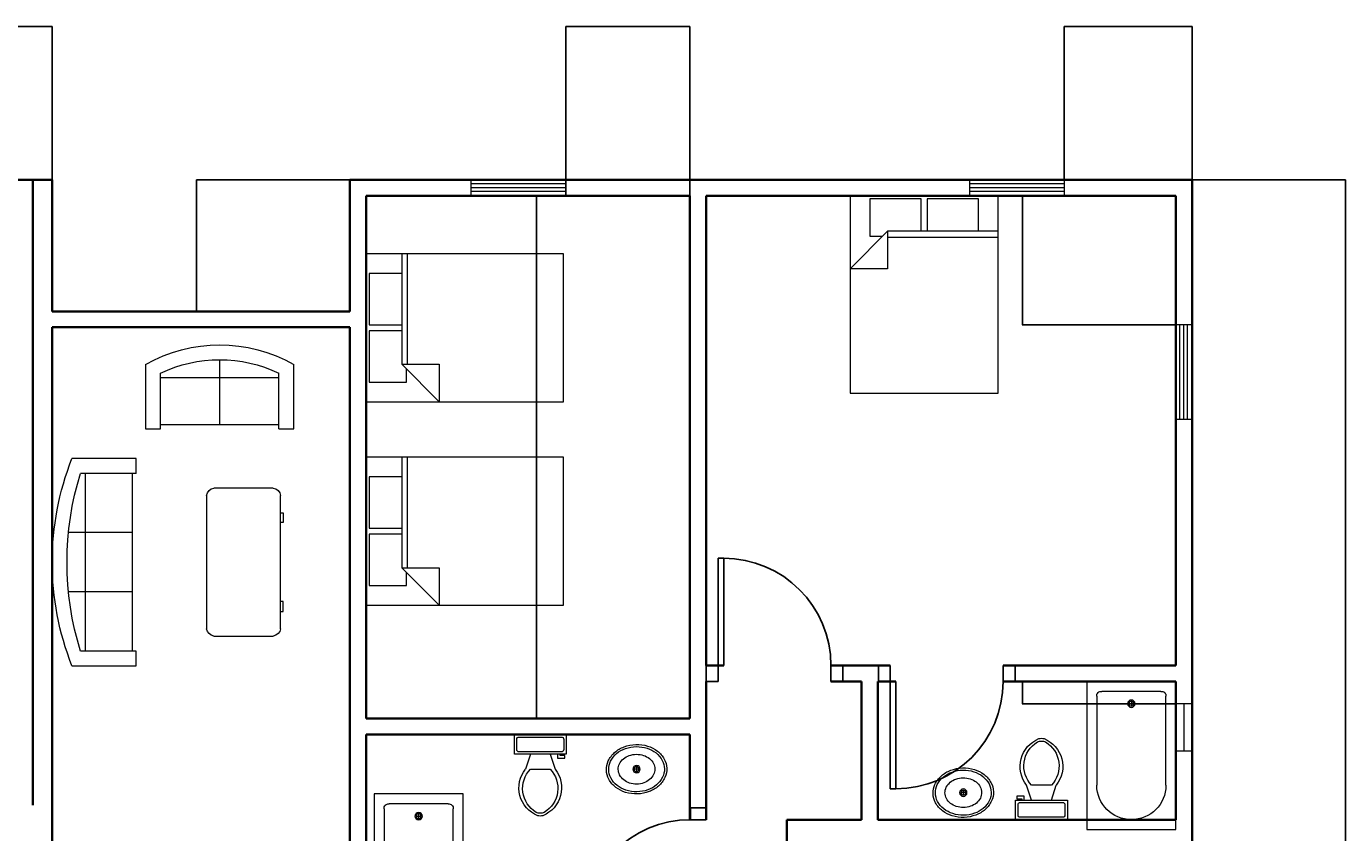
# Model space of a CAD drawing. Units: millimetres. Extents: x 31 to 27050, y -916 to 32407.
# Tile 7 of 7: x 13474 to 27050, y 24108 to 32407. Entities that reach past the tile are written whole.
import ezdxf

# ---------------------------------------------------------------- set-up
doc = ezdxf.new("R2010")
doc.units = ezdxf.units.MM
for name, color, linetype, lineweight in [('A-ANNO-DIMS', 2, 'Continuous', 18), ('A-DOOR', 3, 'Continuous', 25), ('A-FLOR-FIXT', 9, 'Continuous', 18), ('A-FURN', 8, 'Continuous', 13), ('A-GLAZ', 4, 'Continuous', 18), ('A-WALL', 7, 'Continuous', 35)]:
    doc.layers.add(name, color=color, linetype=linetype, lineweight=lineweight)
doc.styles.get("Standard").update_dxf_attribs({"font": 'arial.ttf'})
doc.dimstyles.get("Standard").update_dxf_attribs({"dimtxt": 0.18, "dimasz": 0.18, "dimexe": 0.18, "dimexo": 0.0625, "dimgap": 0.09, "dimtad": 0, "dimtih": 1, "dimtoh": 1, "dimdec": 4, "dimzin": 0, "dimdsep": 46, "dimtxsty": 'Standard', "dimcen": 0.09, "dimadec": 0, "dimazin": 0, "dimtfac": 1, "dimtdec": 4, "dimtofl": 0, "dimtmove": 0, "dimatfit": 3, "dimfxl": 1, "dimtolj": 1, "dimtzin": 0, "dimarcsym": 0})

# ---------------------------------------------------------------- blocks, each defined once
blk = doc.blocks.new('Bath Tub - 26 x 60 in.')
for p, q in [((8, -18), (10, -18)), ((9, -17), (9, -19))]:
    blk.add_line(p, q)
blk.add_lwpolyline([(0, -36), (0, 0), (60, 0), (60, -36)], close=True)
for points in [[(6, -4), (42, -4)], [(4, -30), (4, -6)], [(42, -32), (6, -32)]]:
    blk.add_lwpolyline(points)
for radius in [1.5, 1]:
    blk.add_circle((9, -18), radius)
for centre, radius, start, end in [((5.75, -5.75), 1.767766999999999, 81.86989999999999, 188.1301), ((42, -18), 14, 270, 90), ((5.75, -30.25), 1.767766999999999, 171.8699, 278.1301)]:
    blk.add_arc(centre, radius, start, end)
blk = doc.blocks.new('Sink - Oval top')
for p, q in [((-1, 0), (1, 0)), ((0, 1), (0, -1))]:
    blk.add_line(p, q)
for points in [[(-12.23371880354079, 0.3941914712607968, 0.1176342565883263), (-11.46456229543957, -3.361933235489118, 0.104469279667093), (-8.878748691070427, -6.803541973650567, 0.0900157896014849), (-5.082757700676665, -9.072309807490512, 0.0819199491592185), (-0.3227280122732736, -10.01585280257211, 0.0819199491592091), (4.488169920880977, -9.380701564817912, 0.0900157896014801), (8.422342359155778, -7.36101289847943, 0.1044692796670922), (11.22435122606941, -4.093009071543406, 0.1176342565883338), (12.23371880354091, -0.3941914712607968, 0.1176342565883057), (11.46456229543992, 3.361933235488777, 0.1044692796670849), (8.878748691070427, 6.803541973650567, 0.0900157896014884), (5.082757700676324, 9.072309807490681, 0.0819199491592058), (0.3227280122732736, 10.01585280257211, 0.081919949159207), (-4.488169920880864, 9.380701564817969, 0.0900157896014802), (-8.422342359155778, 7.36101289847943, 0.1044692796670951), (-11.22435122606919, 4.093009071543633, 0.1176342565883402)], [(-11.28627986850119, 0.1590597164737346, 0.1186217001864142), (-10.51590095791209, -3.253161772358112, 0.1046781721811095), (-8.071803350560115, -6.358618019863342, 0.0895620664691738), (-4.537699193222351, -8.366971929609804, 0.0811846988912177), (-0.1289739026695997, -9.15150355811437, 0.0811846988912276), (4.300109150126218, -8.491524865184601, 0.0895620664691798), (7.889406708212618, -6.583562428127606, 0.1046781721811044), (10.42004782883111, -3.548216131892445, 0.1186217001864013), (11.28627986850119, -0.1590597164736209, 0.1186217001863945), (10.51590095791221, 3.253161772357998, 0.1046781721811069), (8.071803350560115, 6.358618019863342, 0.0895620664691756), (4.537699193222124, 8.366971929609917, 0.081184698891216), (0.1289739026695997, 9.151503558114428, 0.0811846988912142), (-4.300109150125877, 8.491524865184829, 0.0895620664691747), (-7.889406708212618, 6.583562428127606, 0.1046781721811045), (-10.42004782883111, 3.548216131892445, 0.1186217001863946)], [(-7.420452389032902, 0.0829876781601797, 0.1182825673856775), (-6.907065465214486, -2.1674649380775, 0.1046074595377274), (-5.294791470712084, -4.209988192029413, 0.0897179636260996), (-2.966599981142508, -5.528122152688069, 0.0814360825277113), (-0.0675135187855176, -6.036810076758797, 0.0814360825277218), (2.84222437824053, -5.593085960977873, 0.0897179636261315), (5.199312936802016, -4.327350491993342, 0.1046074595376878), (6.85686365682659, -2.321395784920355, 0.1182825673856714), (7.420452389033016, -0.0829876781601797, 0.1182825673856961), (6.907065465214486, 2.167464938077614, 0.1046074595377135), (5.294791470712084, 4.209988192029413, 0.0897179636261265), (2.966599981142621, 5.528122152687842, 0.0814360825277426), (0.0675135187855176, 6.036810076758797, 0.0814360825277225), (-2.842224378240644, 5.593085960977873, 0.0897179636261212), (-5.199312936802016, 4.327350491993342, 0.1046074595377049), (-6.856863656826476, 2.321395784920355, 0.1182825673856712)]]:
    blk.add_lwpolyline(points, format="xyb", close=True)
for radius in [1.5, 1]:
    blk.add_circle((0, 0), radius)
blk = doc.blocks.new('Toilet - top')
for p, q in [((9.5, -6), (9.5, -2)), ((-10, -8.5), (-8, -8.5)), ((-10, -9.5), (-10, -8.5)), ((-7, -9.5), (-10, -9.5)), ((-8, -8.5), (-8, -8)), ((-7, -8), (-7, -9.5)), ((-4, -8), (-6, -14)), ((4, -8), (6, -14)), ((4, -14), (-4, -14))]:
    blk.add_line(p, q)
blk.add_lwpolyline([(10.5, -8), (10.5, 0), (-10.5, 0), (-10.5, -8)], close=True)
for points in [[(-9.5, -2), (-9.5, -6)], [(8.5, -1), (-8.5, -1)], [(-8.5, -7), (8.5, -7)]]:
    blk.add_lwpolyline(points)
for centre, radius, start, end in [((-8.625, -1.875), 0.8838834999999999, 81.86989999999999, 188.1301), ((8.625, -1.875), 0.8838834999999999, 351.8699, 98.13009999999998), ((-8.625, -6.125), 0.8838834999999999, 171.869898, 278.1301), ((8.625, -6.125), 0.8838834999999999, 261.8699, 8.130099999999993), ((3.519562435188956, -21.58049502388982), 12.16902005083646, 141.4691096810948, 247.9714346835576), ((4.199957580658807, -21.81740929088453), 11.3291791325804, 136.3677254423718, 238.946823937405), ((-3.519499936778316, -21.58047137067522), 12.16903423757823, 292.0284332733152, 38.53070636800453), ((-4.199890672038477, -21.81738596564128), 11.32918622148567, 301.0530065773863, 43.63209216694732), ((2.09660981727e-05, -27.87646475467881), 4, 245.7318247449371, 294.2681740488959), ((2.09415214183e-05, -28.99996806116075), 4, 254.8605283244437, 285.1394707718433)]:
    blk.add_arc(centre, radius, start, end)
blk = doc.blocks.new('Sofa - Roundback 7 ft.')
for p, q in [((-12.00002, -32.44210000000393), (-12.00003, -6.597100000003898)), ((11.99996999999999, -32.44210000000393), (11.99997999999999, -6.597100000003898)), ((-36.000027, -34.00000000000395), (-36.000027, -11.46960000000396)), ((-35.999844, -13.38190000000397), (35.99979999999999, -13.38190000000397)), ((35.99997999999999, -34.00000000000395), (35.99997999999999, -11.46960000000396)), ((-36.000027, -32.44210000000393), (35.99997999999999, -32.44210000000393))]:
    blk.add_line(p, q)
for points in [[(-36.000027, -34.00000000000395), (-42.000027, -34.00000000000395), (-42.000027, -8.000000000003944)], [(41.99997999999999, -8.000000000003944), (41.99997999999999, -34.00000000000395), (35.99997999999999, -34.00000000000395)]]:
    blk.add_lwpolyline(points)
for centre, radius, start, end in [((0, -114.2500000000039), 114.2500000000039, 68.43141000000072, 111.5686000000006), ((-1.00000000032e-05, -127.1968000000039), 121.1967999999973, 72.72032999999948, 107.2797000000005)]:
    blk.add_arc(centre, radius, start, end)
blk = doc.blocks.new('Sofa - Roundback Loveseat 5 ft.')
for p, q in [((0, -32.44198000000246), (0, -5.999980000002448)), ((-23.99999999999999, -33.99998000000245), (-23.99999999999999, -11.46958000000243)), ((-23.99979999999998, -13.38178000000245), (23.99986, -13.38178000000245)), ((24.00004000000001, -33.99998000000245), (24.00004000000001, -11.46958000000243)), ((-23.99999999999999, -32.44198000000246), (24.00004000000001, -32.44198000000246))]:
    blk.add_line(p, q)
for points in [[(-23.99999999999999, -33.99998000000245), (-29.99999999999999, -33.99998000000245), (-29.99999999999999, -7.999980000002448)], [(30.00004000000001, -7.999980000002448), (30.00004000000001, -33.99998000000245), (24.00004000000001, -33.99998000000245)]]:
    blk.add_lwpolyline(points)
for centre, radius, start, end in [((0, -60.24998000000245), 60.24998000000245, 60.13715000000122, 119.862800000004), ((0, -61.38438000000245), 55.38444000000723, 64.32083000000306, 115.6791999999996)]:
    blk.add_arc(centre, radius, start, end)
blk = doc.blocks.new('Desk - 30 x 60 in.')
for p, q in [((-26.999995, 0), (26.999995, 0)), ((-29.999995, -27), (-29.999995, -3)), ((29.999995, -3), (29.999995, -27)), ((26.999995, -30), (-26.999995, -30)), ((-20.000005, -30), (-20.000005, -31)), ((-20.000005, -31), (-16.000005, -31)), ((-16.000005, -31), (-16.000005, -30)), ((15.999995, -31), (15.999995, -30)), ((19.999995, -31), (15.999995, -31)), ((19.999995, -30), (19.999995, -31))]:
    blk.add_line(p, q)
for centre, radius, start, end in [((-26.499995, -3.5), 3.535534000004229, 98.1300999999916, 171.8698999999352), ((26.499995, -3.5), 3.535533999997753, 8.130102000022115, 81.8698999999439), ((-26.499995, -26.5), 3.535534000000845, 188.1301000000653, 261.8699000000085), ((26.499995, -26.5), 3.535534000004826, 278.1301000000561, 351.8698999999439)]:
    blk.add_arc(centre, radius, start, end)
blk = doc.blocks.new('Bed - Queen')
for p, q in [((0, -80.00003000000002), (0, 0)), ((0, 0), (59.99998999999999, 0)), ((59.99998999999999, 0), (59.99998999999999, -80.00003000000002)), ((7.99999, -1.200000000000017), (28.79998, -1.200000000000017)), ((7.99999, -14.4), (7.99999, -1.200000000000017)), ((28.79998, -1.200000000000017), (28.79998, -14.4)), ((31.19999, -1.200000000000017), (51.99999000000001, -1.200000000000017)), ((31.19999, -14.4), (31.19999, -1.200000000000017)), ((51.99999000000001, -1.200000000000017), (51.99999000000001, -16.4)), ((0, -14.4), (44.79999999999999, -14.4)), ((59.99998999999999, -29.60000000000001), (44.79999999999999, -14.4)), ((44.79999999999999, -14.4), (44.79999999999999, -29.60000000000001)), ((44.79999999999999, -16.80000000000001), (0, -16.80000000000001)), ((51.99999000000001, -16.4), (46.79936, -16.4)), ((44.79999999999999, -29.60000000000001), (59.99998999999999, -29.60000000000001)), ((59.99998999999999, -80.00003000000002), (0, -80.00003000000002))]:
    blk.add_line(p, q)
blk = doc.blocks.new('Window - Wood Frame 36 in. Wide plan')
for p, q in [((0, 6), (0, 0)), ((36, 6), (36, 0)), ((0, 4.5), (36, 4.5)), ((0, 3), (36, 3)), ((0, 1.5), (36, 1.5))]:
    blk.add_line(p, q)
blk = doc.blocks.new('DOOR-SINGLE-1104')
for p, q in [((56.41678681898429, 1104.337341461596), (-7.18501e-11, 1104.337341461596)), ((-7.18501e-11, 1104.337341461596), (-7.18501e-11, 3.638e-12)), ((56.41678681898429, 7.276e-12), (56.41678681898429, 1104.337341461596)), ((-1226.913698425656, -163.8831223050438), (-1226.913698425656, 3.638e-12)), ((-1104.337341461589, 3.638e-12), (-1226.913698425656, 7.276e-12)), ((-1104.337341461589, 3.638e-12), (-1104.337341461589, -163.8831223050438)), ((-7.18501e-11, 3.638e-12), (56.41678681898429, 7.276e-12)), ((56.41678681898429, -163.8831223050438), (56.41678681898429, 3.638e-12)), ((56.41678681898429, 3.638e-12), (178.9931437830519, 3.638e-12)), ((178.9931437830519, 3.638e-12), (178.9931437830519, -163.8831223050438)), ((-1104.337341461589, -163.8831223050438), (-1226.913698425656, -163.8831223050438)), ((178.9931437830519, -163.8831223050438), (56.41678681898429, -163.8831223050438))]:
    blk.add_line(p, q)
blk.add_arc((0, 3.638e-12), 1104.337341461589, 90, 180)
blk = doc.blocks.new('WIN-BATH-482')
for p, q in [((0, 3.638e-12), (-168.350650710694, 3.638e-12)), ((-84.17532535534633, -482.3297634273148), (-84.17532535534701, 3.638e-12)), ((-168.350650710694, -482.3297634273148), (1.3642e-12, -482.3297634273148))]:
    blk.add_line(p, q)
blk = doc.blocks.new('*D47')
at = {"layer": 'A-ANNO-DIMS', "color": 0, "lineweight": -2, "transparency": 16777216}
for p, q in [((25471.21116800002, 30827.53125900001), (27050.32866800003, 30827.53125900001)), ((27050.14866800003, 30827.35125900001), (27050.14866800003, 15745.77166202933)), ((27050.14866800004, 663.8281360000004), (27050.14866800003, 15745.40773297067)), ((25471.21116800002, 663.6481360000002), (27050.32866800003, 663.6481360000004))]:
    blk.add_line(p, q, dxfattribs=at)
at = {"layer": 'A-ANNO-DIMS', "color": 0, "transparency": 16777216}
for points in [[(27050.11866800003, 30827.35125900001), (27050.17866800003, 30827.35125900001), (27050.14866800003, 30827.53125900001)], [(27050.11866800004, 663.8281360000004), (27050.17866800004, 663.8281360000004), (27050.14866800004, 663.6481360000004)]]:
    blk.add_solid(points, dxfattribs=at)
at = {"layer": 'Defpoints', "color": 0, "transparency": 16777216}
for p in [(25471.14866800002, 30827.53125900001), (27050.14866800003, 30827.53125900001), (25471.14866800002, 663.6481360000002)]:
    blk.add_point(p, dxfattribs=at)
at = {"layer": 'A-ANNO-DIMS', "color": 0, "transparency": 16777216, "insert": (27050.14866800003, 15745.58969749999), "char_height": 0.18, "attachment_point": 5}
blk.add_mtext('\\A1;30164', dxfattribs=at)
blk = doc.blocks.new('*D51')
at = {"layer": 'A-ANNO-DIMS', "color": 0, "lineweight": -2, "transparency": 16777216}
for p, q in [((13340.585333, 30827.593759), (13340.585333, 32406.711259)), ((13340.765333, 32406.531259), (13540.29317065348, 32406.531259)), ((13740.405333, 32406.531259), (13540.87749534652, 32406.531259)), ((13740.585333, 30827.593759), (13740.585333, 32406.711259))]:
    blk.add_line(p, q, dxfattribs=at)
at = {"layer": 'A-ANNO-DIMS', "color": 0, "transparency": 16777216}
for points in [[(13340.765333, 32406.561259), (13340.765333, 32406.501259), (13340.585333, 32406.531259)], [(13740.405333, 32406.561259), (13740.405333, 32406.501259), (13740.585333, 32406.531259)]]:
    blk.add_solid(points, dxfattribs=at)
at = {"layer": 'Defpoints', "color": 0, "transparency": 16777216}
for p in [(13740.585333, 32406.531259), (13340.585333, 30827.531259), (13740.585333, 30827.531259)]:
    blk.add_point(p, dxfattribs=at)
at = {"layer": 'A-ANNO-DIMS', "color": 0, "transparency": 16777216, "insert": (13540.585333, 32406.531259), "char_height": 0.18, "attachment_point": 5}
blk.add_mtext('\\A1;400', dxfattribs=at)
blk = doc.blocks.new('*D63')
at = {"layer": 'A-ANNO-DIMS', "color": 0, "lineweight": -2, "transparency": 16777216}
for p, q in [((20302.73551700001, 30663.64813600002), (18723.61801700001, 30663.64813600002)), ((18723.79801700001, 30663.46813600001), (18723.79801700001, 27973.32699502935)), ((18723.79801700001, 25282.82192500002), (18723.79801700001, 27972.96306597068)), ((20302.73551700001, 25282.64192500002), (18723.61801700001, 25282.64192500002))]:
    blk.add_line(p, q, dxfattribs=at)
at = {"layer": 'A-ANNO-DIMS', "color": 0, "transparency": 16777216}
for points in [[(18723.76801700001, 30663.46813600001), (18723.82801700001, 30663.46813600001), (18723.79801700001, 30663.64813600002)], [(18723.76801700001, 25282.82192500002), (18723.82801700001, 25282.82192500002), (18723.79801700001, 25282.64192500002)]]:
    blk.add_solid(points, dxfattribs=at)
at = {"layer": 'Defpoints', "color": 0, "transparency": 16777216}
for p in [(18723.79801700001, 30663.64813600002), (20302.79801700001, 30663.64813600002), (20302.79801700001, 25282.64192500002)]:
    blk.add_point(p, dxfattribs=at)
at = {"layer": 'A-ANNO-DIMS', "color": 0, "transparency": 16777216, "insert": (18723.79801700002, 27973.1450305), "char_height": 0.18, "attachment_point": 5}
blk.add_mtext('\\A1;5381', dxfattribs=at)
blk = doc.blocks.new('*D76')
at = {"layer": 'A-ANNO-DIMS', "color": 0, "lineweight": -2, "transparency": 16777216}
for p, q in [((24155.62247, 30827.593759), (24155.62247, 32406.711259)), ((24155.80247, 32406.531259), (24812.92973680354, 32406.531259)), ((25470.968668, 32406.531259), (24813.84140119645, 32406.531259)), ((25471.148668, 30827.593759), (25471.148668, 32406.711259))]:
    blk.add_line(p, q, dxfattribs=at)
at = {"layer": 'A-ANNO-DIMS', "color": 0, "transparency": 16777216}
for points in [[(24155.80247, 32406.561259), (24155.80247, 32406.501259), (24155.62247, 32406.531259)], [(25470.968668, 32406.561259), (25470.968668, 32406.501259), (25471.148668, 32406.531259)]]:
    blk.add_solid(points, dxfattribs=at)
at = {"layer": 'Defpoints', "color": 0, "transparency": 16777216}
for p in [(24155.62247, 32406.531259), (24155.62247, 30827.531259), (25471.148668, 30827.531259)]:
    blk.add_point(p, dxfattribs=at)
at = {"layer": 'A-ANNO-DIMS', "color": 0, "transparency": 16777216, "insert": (24813.385569, 32406.531259), "char_height": 0.18, "attachment_point": 5}
blk.add_mtext('\\A1;1315.5', dxfattribs=at)
blk = doc.blocks.new('*D77')
at = {"layer": 'A-ANNO-DIMS', "color": 0, "lineweight": -2, "transparency": 16777216}
for p, q in [((19025.756761, 30664.919965), (19025.756761, 32406.711259)), ((19025.936761, 32406.531259), (19663.92708886358, 32406.531259)), ((20302.618017, 32406.531259), (19664.62768913643, 32406.531259)), ((20302.798017, 30663.710636), (20302.798017, 32406.711259))]:
    blk.add_line(p, q, dxfattribs=at)
at = {"layer": 'A-ANNO-DIMS', "color": 0, "transparency": 16777216}
for points in [[(19025.936761, 32406.561259), (19025.936761, 32406.501259), (19025.756761, 32406.531259)], [(20302.618017, 32406.561259), (20302.618017, 32406.501259), (20302.798017, 32406.531259)]]:
    blk.add_solid(points, dxfattribs=at)
at = {"layer": 'Defpoints', "color": 0, "transparency": 16777216}
for p in [(19025.756761, 32406.531259), (19025.756761, 30664.857465), (20302.798017, 30663.648136)]:
    blk.add_point(p, dxfattribs=at)
at = {"layer": 'A-ANNO-DIMS', "color": 0, "transparency": 16777216, "insert": (19664.277389, 32406.531259), "char_height": 0.18, "attachment_point": 5}
blk.add_mtext('\\A1;1277', dxfattribs=at)
blk = doc.blocks.new('*D80')
at = {"layer": 'A-ANNO-DIMS', "color": 0, "lineweight": -2, "transparency": 16777216}
for p, q in [((25302.73551700001, 30663.64813600002), (23723.61801700002, 30663.64813600001)), ((23723.79801700001, 30663.46813600001), (23723.79801700001, 29999.37617352935)), ((23723.79801700001, 29334.92028200001), (23723.79801700001, 29999.01224447068)), ((25302.73551700001, 29334.74028200001), (23723.61801700002, 29334.74028200001))]:
    blk.add_line(p, q, dxfattribs=at)
at = {"layer": 'A-ANNO-DIMS', "color": 0, "transparency": 16777216}
for points in [[(23723.76801700002, 30663.46813600001), (23723.82801700001, 30663.46813600001), (23723.79801700001, 30663.64813600001)], [(23723.76801700002, 29334.92028200001), (23723.82801700001, 29334.92028200001), (23723.79801700001, 29334.74028200001)]]:
    blk.add_solid(points, dxfattribs=at)
at = {"layer": 'Defpoints', "color": 0, "transparency": 16777216}
for p in [(23723.79801700001, 30663.64813600001), (25302.79801700002, 30663.64813600002), (25302.79801700002, 29334.74028200001)]:
    blk.add_point(p, dxfattribs=at)
at = {"layer": 'A-ANNO-DIMS', "color": 0, "transparency": 16777216, "insert": (23723.79801700002, 29999.194209), "char_height": 0.18, "attachment_point": 5}
blk.add_mtext('\\A1;1329', dxfattribs=at)
blk = doc.blocks.new('*D85')
at = {"layer": 'A-ANNO-DIMS', "color": 0, "lineweight": -2, "transparency": 16777216}
for p, q in [((25302.73551700001, 25663.64813600002), (23723.61801700002, 25663.64813600001)), ((23723.79801700001, 25663.46813600001), (23723.79801700001, 25548.22429702935)), ((23723.79801700001, 25432.61652900001), (23723.79801700001, 25547.86036797068)), ((25302.73551700001, 25432.43652900001), (23723.61801700002, 25432.43652900001))]:
    blk.add_line(p, q, dxfattribs=at)
at = {"layer": 'A-ANNO-DIMS', "color": 0, "transparency": 16777216}
for points in [[(23723.76801700002, 25663.46813600001), (23723.82801700001, 25663.46813600001), (23723.79801700001, 25663.64813600001)], [(23723.76801700002, 25432.61652900001), (23723.82801700001, 25432.61652900001), (23723.79801700001, 25432.43652900001)]]:
    blk.add_solid(points, dxfattribs=at)
at = {"layer": 'Defpoints', "color": 0, "transparency": 16777216}
for p in [(23723.79801700001, 25663.64813600001), (25302.79801700002, 25663.64813600002), (25302.79801700002, 25432.43652900001)]:
    blk.add_point(p, dxfattribs=at)
at = {"layer": 'A-ANNO-DIMS', "color": 0, "transparency": 16777216, "insert": (23723.79801700002, 25548.0423325), "char_height": 0.18, "attachment_point": 5}
blk.add_mtext('\\A1;231.2', dxfattribs=at)
blk = doc.blocks.new('*D86')
at = {"layer": 'A-ANNO-DIMS', "color": 0, "lineweight": -2, "transparency": 16777216}
for p, q in [((16802.73551700001, 30827.53125900001), (15223.61801700001, 30827.53125900001)), ((15223.79801700001, 30827.35125900001), (15223.79801700001, 30150.57652452934)), ((15223.79801700001, 29473.43786100002), (15223.79801700001, 30150.21259547068)), ((16802.73551700001, 29473.25786100001), (15223.61801700001, 29473.25786100001))]:
    blk.add_line(p, q, dxfattribs=at)
at = {"layer": 'A-ANNO-DIMS', "color": 0, "transparency": 16777216}
for points in [[(15223.76801700001, 30827.35125900001), (15223.82801700001, 30827.35125900001), (15223.79801700001, 30827.53125900001)], [(15223.76801700001, 29473.43786100002), (15223.82801700001, 29473.43786100002), (15223.79801700001, 29473.25786100001)]]:
    blk.add_solid(points, dxfattribs=at)
at = {"layer": 'Defpoints', "color": 0, "transparency": 16777216}
for p in [(15223.79801700001, 30827.53125900001), (16802.79801700001, 30827.53125900001), (16802.79801700001, 29473.25786100001)]:
    blk.add_point(p, dxfattribs=at)
at = {"layer": 'A-ANNO-DIMS', "color": 0, "transparency": 16777216, "insert": (15223.79801700002, 30150.39456), "char_height": 0.18, "attachment_point": 5}
blk.add_mtext('\\A1;1354.3', dxfattribs=at)

msp = doc.modelspace()

# ---------------------------------------------------------------- linework, layer by layer
at = {"layer": 'A-DOOR'}
for p, q in [((20593.7250250705, 26931.86860013333), (20593.7250250705, 26931.86860013333)), ((20471.14866810643, 25827.53125867173), (20593.7250250705, 25827.53125867174)), ((20593.7250250705, 25663.64813636669), (20471.14866810643, 25663.64813636669))]:
    msp.add_line(p, q, dxfattribs=at)
at = {"layer": 'A-WALL'}
for p, q in [((13540.58533261045, 30827.53125867174), (13340.58533261045, 30827.53125867174)), ((13540.58533261045, 30744.3803777756), (13540.58533261045, 30827.53125867173)), ((13540.58533261045, 30827.53125867174), (13740.58533261045, 30827.53125867174)), ((13540.58533261045, 30744.3803777756), (13540.58533261045, 30827.53125867173)), ((13740.58533261045, 30744.3803777756), (13740.58533261045, 30827.53125867173)), ((16802.79801739574, 30827.53125867173), (21890.58533261044, 30827.53125867173)), ((16802.79801739574, 30663.64813636668), (16802.79801739574, 30827.53125867173)), ((25390.58533261046, 30827.53125867173), (16890.58533261045, 30827.53125867173)), ((25471.14866810643, 30827.53125867173), (25352.99341396501, 30827.53125867173)), ((25471.14866810643, 30744.38037777559), (25471.14866810643, 30827.53125867173)), ((13540.58533261045, 29390.10698055507), (13540.58533261045, 30744.3803777756)), ((13540.58533261045, 29390.10698055507), (13540.58533261045, 30744.3803777756)), ((13740.58533261045, 29473.25786145121), (13740.58533261045, 30744.3803777756)), ((25471.14866810643, 19025.43572389214), (25471.14866810643, 30744.3803777756)), ((25471.14866810643, 30744.38037777559), (25471.14866810643, 19106.16796530105)), ((25471.14866810643, 30744.38037777559), (25471.14866810643, 25744.38037777559)), ((16802.79801739574, 29473.25786145121), (16802.79801739574, 30663.64813636668)), ((16971.14866810643, 30663.64813636668), (20302.79801739574, 30663.64813636668)), ((20302.79801739574, 30663.64813636669), (16971.14866810643, 30663.64813636669)), ((16971.14866810643, 25282.64192458121), (16971.14866810643, 30663.64813636668)), ((20302.79801739574, 30663.64813636668), (20302.79801739574, 25282.64192458121)), ((20471.14866810643, 30663.64813636668), (21890.58533261044, 30663.64813636668)), ((25302.79801739574, 30663.64813636668), (20471.14866810643, 30663.64813636668)), ((20471.14866810643, 30663.64813636669), (20471.14866810643, 25827.53125867174)), ((25302.79801739574, 25827.53125867173), (25302.79801739574, 30663.64813636667)), ((25302.79801739574, 30663.64813636668), (25302.79801739574, 25827.53125867173)), ((25302.79801739574, 30663.64813636668), (25302.79801739574, 25827.53125867174)), ((16802.79801739574, 29473.25786145121), (13740.58533261045, 29473.25786145121)), ((13540.58533261045, 24390.10698055507), (13540.58533261045, 29390.10698055507)), ((13540.58533261045, 24390.10698055507), (13540.58533261045, 29390.10698055507)), ((13740.58533261045, 29309.37473914617), (13740.58533261045, 24473.25786145121)), ((16802.79801739574, 29309.37473914616), (13740.58533261045, 29309.37473914617)), ((16802.79801739574, 24473.25786145121), (16802.79801739574, 29309.37473914616)), ((20650.14181188956, 25827.53125867174), (20471.14866810643, 25827.53125867173)), ((22364.9602385284, 25827.53125867174), (21754.47915335108, 25827.53125867173)), ((25302.79801739574, 25827.53125867173), (23525.71436680897, 25827.53125867174)), ((20471.14866810643, 25663.64813636668), (20471.14866810643, 24240.83204693513)), ((22066.96169576355, 25663.64813636669), (21754.47915335108, 25663.64813636669)), ((22066.96169576355, 24240.63568990879), (22066.96169576355, 25663.64813636669)), ((22421.37702534746, 25663.64813636668), (22235.31234647424, 25663.64813636669)), ((22235.31234647424, 24240.63568990878), (22235.31234647424, 25663.64813636669)), ((25302.79801739574, 25663.64813636668), (23525.71436680897, 25663.64813636669)), ((25302.79801739574, 24240.63568990878), (25302.79801739574, 25663.64813636669)), ((25302.79801739574, 25663.64813636668), (25302.79801739574, 24240.63568990879)), ((20302.79801739574, 25282.64192458121), (16971.14866810643, 25282.64192458121)), ((16971.14866810643, 22919.96829640664), (16971.14866810643, 25117.33256545015)), ((16971.14866810643, 25117.33256545015), (20302.79801739574, 25117.33256545015)), ((20302.79801739574, 25117.33256545015), (20302.79801739574, 24240.82301034324)), ((13740.58533261045, 24473.25786145121), (13740.58533261045, 24309.37473914616)), ((16802.79801739574, 24473.25786145121), (16802.79801739574, 24309.37473914615)), ((13740.58533261045, 18102.01062910059), (13740.58533261045, 24309.37473914616)), ((16802.79801739574, 18469.90100734673), (16802.79801739574, 24309.37473914615)), ((21387.2503044143, 24240.63568990878), (21299.46298919959, 24240.63568990879)), ((21299.46298919959, 24240.63568990879), (21299.46298919959, 24157.48480901264)), ((21387.2503044143, 24240.63568990878), (22066.96169576355, 24240.63568990878)), ((22235.31234647424, 24240.63568990878), (25302.79801739574, 24240.63568990878)), ((21299.46298919959, 22535.9107124077), (21299.46298919959, 24157.48480901264))]:
    msp.add_line(p, q, dxfattribs=at)

# ---------------------------------------------------------------- block references
at = {"layer": 'A-DOOR', "extrusion": (0, 0, -1), "zscale": -1}
msp.add_blockref('DOOR-SINGLE-1104', (-20650.14181188949, 25827.53125867173), dxfattribs=at)
at = {"layer": 'A-DOOR', "rotation": 180}
msp.add_blockref('DOOR-SINGLE-1104', (22421.37702534739, 25663.6481363667), dxfattribs=at)
at = {"layer": 'A-DOOR', "extrusion": (0, 0, -1), "zscale": -1, "rotation": 270.0000000000002}
msp.add_blockref('DOOR-SINGLE-1104', (-20307.2655458014, 23136.49470547354), dxfattribs=at)
at = {"layer": 'A-FLOR-FIXT', "xscale": -25.4, "yscale": 25.4, "zscale": 25.4}
for name, p, rotation in [('Bath Tub - 26 x 60 in.', (24388.39801739574, 25663.64813636669), 90), ('Toilet - top', (23920.52980656935, 24240.63568990878), 180), ('Bath Tub - 26 x 60 in.', (17053.83772899901, 24506.11473923286), 90)]:
    msp.add_blockref(name, p, dxfattribs=dict(at, rotation=rotation))
for name, p in [('Toilet - top', (18762.63376664123, 25117.33256545015)), ('Sink - Oval top', (19753.85322183833, 24760.78106746359)), ('Sink - Oval top', (23116.00565271956, 24519.45474699098))]:
    msp.add_blockref(name, p, dxfattribs=at)
at = {"layer": 'A-FURN', "xscale": -25.4, "yscale": 25.4, "zscale": 25.4}
for name, p in [('Bed - Queen', (23474.93713847067, 30663.64813636668)), ('Sofa - Roundback Loveseat 5 ft.', (15463.57834507332, 29128.39471993013))]:
    msp.add_blockref(name, p, dxfattribs=at)
at = {"layer": 'A-FURN', "xscale": -25.4, "yscale": 25.4, "zscale": 25.4, "rotation": 90}
for name, p in [('Bed - Queen', (16971.14866810643, 30066.85799248087)), ('Bed - Queen', (16971.14866810643, 27973.14503047395)), ('Sofa - Roundback 7 ft.', (13740.58533261045, 26891.31630029868)), ('Desk - 30 x 60 in.', (15328.78238791416, 26892.70491289827))]:
    msp.add_blockref(name, p, dxfattribs=at)
at = {"layer": 'A-GLAZ', "xscale": -27.11229900122799, "yscale": 27.11229900122799, "zscale": 27.11229900122799}
for p in [(19025.75676052496, 30664.85746466437), (24155.62246971748, 30664.85746466437)]:
    msp.add_blockref('Window - Wood Frame 36 in. Wide plan', p, dxfattribs=at)
at = {"layer": 'A-GLAZ', "xscale": -27.11229900122799, "yscale": 27.11229900122799, "zscale": 27.11229900122799, "rotation": 270}
msp.add_blockref('Window - Wood Frame 36 in. Wide plan', (25302.79801739574, 28358.69751835588), dxfattribs=at)
at = {"layer": 'A-GLAZ', "rotation": 180}
msp.add_blockref('WIN-BATH-482', (25302.79801739574, 24950.10676542021), dxfattribs=at)

# ---------------------------------------------------------------- dimensions: what is measured, and where the dimension line sits
at = {"layer": 'A-ANNO-DIMS'}
for base, p1, p2, override, picture, middle in [((13740.585333, 32406.531259), (13340.585333, 30827.531259), (13740.585333, 30827.531259), {"dimdec": 0, "dimlfac": 1, "dimrnd": 0, "dimzin": 0, "dimdsep": 46, "dimlunit": 2}, '*D51', (13540.585333, 32406.531259)), ((19025.756761, 32406.531259), (20302.798017, 30663.648136), (19025.756761, 30664.857465), {"dimdec": 0, "dimlfac": 1, "dimrnd": 0, "dimzin": 0, "dimdsep": 46, "dimlunit": 2}, '*D77', (19664.277389, 32406.531259)), ((24155.62247, 32406.531259), (25471.148668, 30827.531259), (24155.62247, 30827.531259), {"dimdec": 1, "dimlfac": 1, "dimrnd": 0, "dimzin": 0, "dimdsep": 46, "dimlunit": 2}, '*D76', (24813.385569, 32406.531259))]:
    dim = msp.add_linear_dim(base=base, p1=p1, p2=p2, dimstyle='Standard', override=override, dxfattribs=at)
    dim.commit()
    dim.dimension.update_dxf_attribs({"geometry": picture, "text_midpoint": middle})
for base, p1, p2, override, picture, middle in [((15223.79801700001, 30827.53125900001), (16802.798017, 29473.257861), (16802.798017, 30827.531259), {"dimdec": 1, "dimlfac": 1, "dimrnd": 0, "dimzin": 0, "dimdsep": 46, "dimlunit": 2}, '*D86', (15223.79801700002, 30150.39456)), ((27050.14866800003, 30827.53125900001), (25471.148668, 663.648136), (25471.148668, 30827.531259), {"dimdec": 0, "dimlfac": 1, "dimrnd": 0, "dimzin": 0, "dimdsep": 46, "dimlunit": 2}, '*D47', (27050.14866800003, 15745.58969749999)), ((18723.79801700001, 30663.64813600002), (20302.798017, 25282.641925), (20302.798017, 30663.648136), {"dimdec": 0, "dimlfac": 1, "dimrnd": 0, "dimzin": 0, "dimdsep": 46, "dimlunit": 2}, '*D63', (18723.79801700002, 27973.1450305)), ((23723.79801700001, 30663.64813600001), (25302.798017, 29334.740282), (25302.798017, 30663.648136), {"dimdec": 0, "dimlfac": 1, "dimrnd": 0, "dimzin": 0, "dimdsep": 46, "dimlunit": 2}, '*D80', (23723.79801700002, 29999.194209)), ((23723.79801700001, 25663.64813600001), (25302.798017, 25432.436529), (25302.798017, 25663.648136), {"dimdec": 1, "dimlfac": 1, "dimrnd": 0, "dimzin": 0, "dimdsep": 46, "dimlunit": 2}, '*D85', (23723.79801700002, 25548.0423325))]:
    dim = msp.add_linear_dim(base=base, p1=p1, p2=p2, angle=90, dimstyle='Standard', override=override, dxfattribs=at)
    dim.commit()
    dim.dimension.update_dxf_attribs({"geometry": picture, "text_midpoint": middle})

doc.saveas('drawing.dxf')
